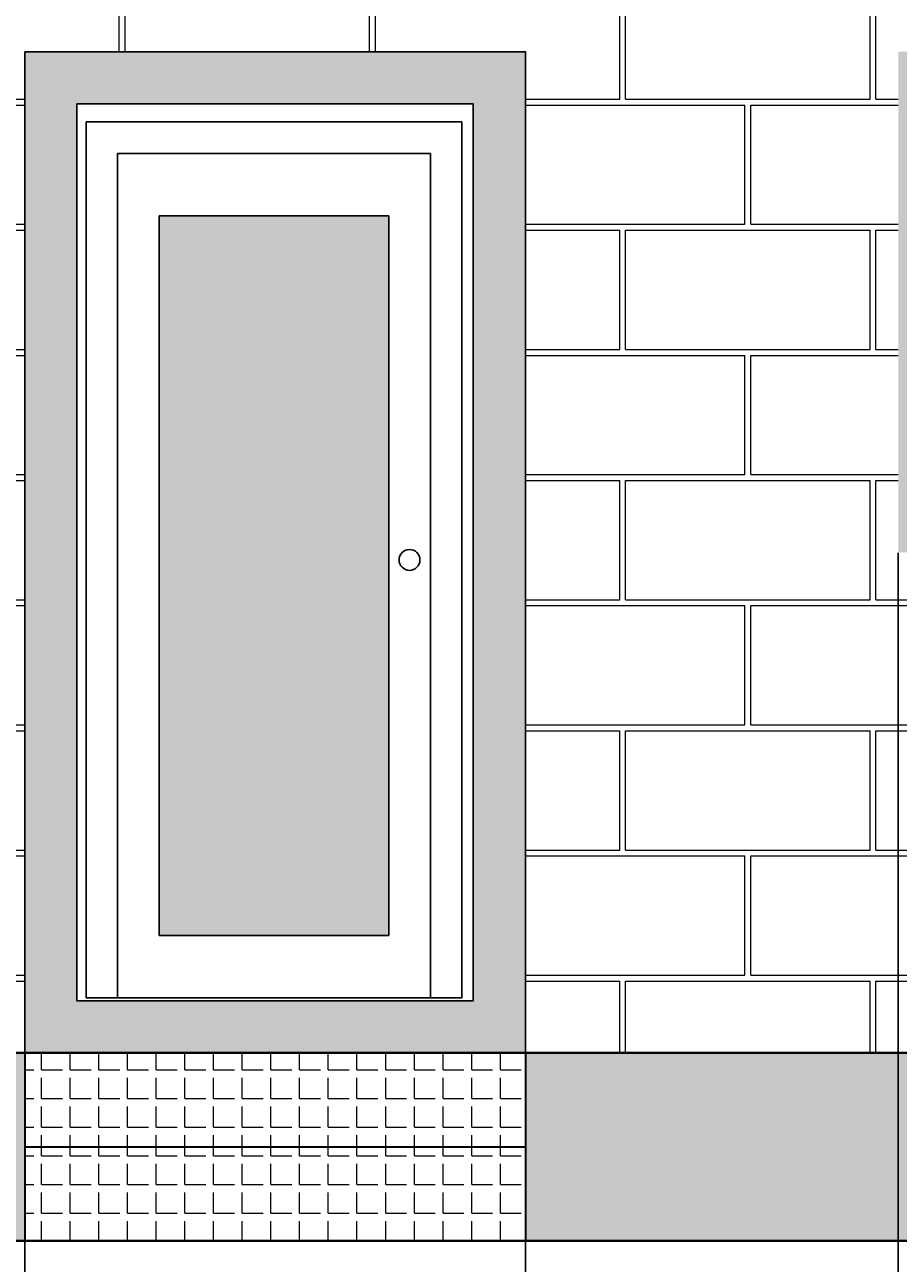
# Model space of a CAD drawing. Units: inches. Extents: x -301 to 715, y -607 to 364.
# Tile 135 of 141: x 413 to 497, y -510 to -391. Entities that reach past the tile are written whole.
import ezdxf

# ---------------------------------------------------------------- set-up
doc = ezdxf.new("R2010")
doc.units = ezdxf.units.IN
doc.header["$MEASUREMENT"] = 0
for name, color, linetype, lineweight in [('A-ANNO-DIMS', 2, 'Continuous', 18), ('A-DOOR', 4, 'Continuous', 25), ('A-ELEV', 220, 'Continuous', 30), ('A-ELEV-PATT', 4, 'Continuous', 13)]:
    doc.layers.add(name, color=color, linetype=linetype, lineweight=lineweight)
doc.styles.get("Standard").update_dxf_attribs({"font": 'arial.ttf'})
doc.dimstyles.get("Standard").update_dxf_attribs({"dimtxt": 0.18, "dimasz": 0.18, "dimexe": 0.18, "dimexo": 0.0625, "dimgap": 0.09, "dimtad": 0, "dimtih": 1, "dimtoh": 1, "dimdec": 1, "dimzin": 0, "dimdsep": 46, "dimlunit": 4, "dimtxsty": 'Standard', "dimcen": 0.09, "dimclrd": 3, "dimclre": 4, "dimclrt": 6, "dimadec": 0, "dimazin": 0, "dimtfac": 1, "dimtdec": 1, "dimtofl": 0, "dimtmove": 0, "dimatfit": 3, "dimfxl": 1, "dimtfill": 2, "dimtfillclr": 51, "dimtolj": 1, "dimtzin": 0, "dimarcsym": 0})

# ---------------------------------------------------------------- blocks, each defined once
blk = doc.blocks.new('*U31')
blk.add_lwpolyline([(3.12, 0.01), (0.12, 0.01), (0.12, 84.01), (36.12, 84.01), (36.12, 0.01), (33.12, 0.01)])
for points in [[(33.12, 80.99), (33.12, 0.01), (3.12, 0.01), (3.12, 80.99)], [(29.12, 6.01), (29.12, 74.99), (7.12, 74.99), (7.12, 6.01)]]:
    blk.add_lwpolyline(points, close=True)
blk.add_circle((31.12, 42.01), 1)
blk = doc.blocks.new('*D197')
at = {"layer": 'A-ANNO-DIMS', "color": 4, "lineweight": -2, "transparency": 16777216}
for p, q in [((413.02, -489.61), (413.02, -606.79)), ((461.02, -489.61), (461.02, -606.79))]:
    blk.add_line(p, q, dxfattribs=at)
at = {"layer": 'A-ANNO-DIMS', "color": 3, "lineweight": -2, "transparency": 16777216}
for p, q in [((413.2, -606.61), (436.68, -606.61)), ((460.84, -606.61), (437.35, -606.61))]:
    blk.add_line(p, q, dxfattribs=at)
at = {"layer": 'A-ANNO-DIMS', "color": 3, "transparency": 16777216}
for points in [[(413.2, -606.58), (413.2, -606.64), (413.02, -606.61)], [(460.84, -606.58), (460.84, -606.64), (461.02, -606.61)]]:
    blk.add_solid(points, dxfattribs=at)
at = {"layer": 'Defpoints', "color": 0, "transparency": 16777216}
for p in [(413.02, -489.55), (461.02, -489.55), (461.02, -606.61)]:
    blk.add_point(p, dxfattribs=at)
at = {"layer": 'A-ANNO-DIMS', "color": 6, "transparency": 16777216, "insert": (437.02, -606.61), "char_height": 0.18, "attachment_point": 5, "bg_fill": 1, "box_fill_scale": 1.25, "bg_fill_color": 51, "bg_fill_transparency": 0}
blk.add_mtext('\\A1;4\'-0"', dxfattribs=at)
blk = doc.blocks.new('*D198')
at = {"layer": 'A-ANNO-DIMS', "color": 4, "lineweight": -2, "transparency": 16777216}
for p, q in [((496.77, -441.61), (496.77, -606.79)), ((461.02, -489.61), (461.02, -606.79))]:
    blk.add_line(p, q, dxfattribs=at)
at = {"layer": 'A-ANNO-DIMS', "color": 3, "lineweight": -2, "transparency": 16777216}
for p, q in [((461.2, -606.61), (478.56, -606.61)), ((496.59, -606.61), (479.22, -606.61))]:
    blk.add_line(p, q, dxfattribs=at)
at = {"layer": 'A-ANNO-DIMS', "color": 3, "transparency": 16777216}
for points in [[(461.2, -606.58), (461.2, -606.64), (461.02, -606.61)], [(496.59, -606.58), (496.59, -606.64), (496.77, -606.61)]]:
    blk.add_solid(points, dxfattribs=at)
at = {"layer": 'Defpoints', "color": 0, "transparency": 16777216}
for p in [(496.77, -441.55), (461.02, -489.55), (496.77, -606.61)]:
    blk.add_point(p, dxfattribs=at)
at = {"layer": 'A-ANNO-DIMS', "color": 6, "transparency": 16777216, "insert": (478.89, -606.61), "char_height": 0.18, "attachment_point": 5, "bg_fill": 1, "box_fill_scale": 1.25, "bg_fill_color": 51, "bg_fill_transparency": 0}
blk.add_mtext('\\A1;3\'-0"', dxfattribs=at)

msp = doc.modelspace()

# ---------------------------------------------------------------- hatches: boundary and pattern name
at = {"layer": 'A-ELEV-PATT'}
h = msp.add_hatch(color=256, dxfattribs=at)
h.dxf.hatch_style = 1
h.paths.add_polyline_path([(591.52, -363.55), (254.02, -363.55), (254.02, -369.55), (591.52, -369.55)])
h.paths.add_polyline_path([(461.02, -393.55), (413.02, -393.55), (413.02, -489.55), (461.02, -489.55)])
h.paths.add_polyline_path([(456.02, -398.55), (456.02, -484.55), (418.02, -484.55), (418.02, -398.55)], flags=16)
h.paths.add_polyline_path([(546.77, -393.55), (496.77, -393.55), (496.77, -441.55), (546.77, -441.55)])
h.paths.add_polyline_path([(501.77, -398.55), (541.77, -398.55), (541.77, -436.55), (501.77, -436.55)], flags=16)
h.paths.add_polyline_path([(360.02, -393.55), (310.02, -393.55), (310.02, -441.55), (360.02, -441.55)])
h.paths.add_polyline_path([(355.02, -398.55), (355.02, -436.55), (315.02, -436.55), (315.02, -398.55)], flags=16)
h = msp.add_hatch(dxfattribs=at)
h.set_pattern_fill('AR-B816C', color=256, scale=1.5)
h.set_pattern_definition([(0, (458.621, 9.325), (12, 12), [23.4375, -0.5625]), (0, (446.621, 9.887), (12, 12), [23.4375, -0.5625]), (90, (458.621, 9.325), (-12, 12), [-12.5625, 11.4375]), (90, (458.059, 9.325), (-12, 12), [-12.5625, 11.4375])])
h.paths.add_polyline_path([(254.02, -489.55), (413.02, -489.55), (413.02, -393.55), (461.02, -393.55), (461.02, -489.55), (591.52, -489.55), (591.52, -369.55), (254.02, -369.55)])
h.paths.add_polyline_path([(310.02, -393.55), (360.02, -393.55), (360.02, -441.55), (310.02, -441.55)], flags=16)
h.paths.add_polyline_path([(315.02, -398.55), (355.02, -398.55), (355.02, -436.55), (315.02, -436.55)], flags=0)
h.paths.add_polyline_path([(496.77, -393.55), (546.77, -393.55), (546.77, -441.55), (496.77, -441.55)], flags=16)
h.paths.add_polyline_path([(501.77, -398.55), (541.77, -398.55), (541.77, -436.55), (501.77, -436.55)], flags=0)
h = msp.add_hatch(color=256, dxfattribs=at)
h.dxf.hatch_style = 1
h.paths.add_polyline_path([(425.92, -478.28), (447.92, -478.28), (447.92, -409.3), (425.92, -409.3)])
h = msp.add_hatch(dxfattribs=at)
h.set_pattern_fill('AR-CONC', color=256, scale=2)
h.set_pattern_definition([(50, (458.621, 9.325), (14.3452, -1.25504), [1.5, -16.5]), (355, (458.621, 9.325), (-2.77503, 15.04384), [1.2, -13.2]), (100.4514, (459.817, 9.22), (11.57018, 13.7888), [1.2748, -14.02284]), (46.1842, (458.621, 13.325), (21.3448, -3.3104), [2.25, -24.75]), (96.6356, (460.4, 13.049), (18.69324, 19.4824), [1.9122, -21.0343]), (351.184, (458.62, 13.325), (18.6932, 19.4824), [1.8, -19.8]), (21, (460.621, 12.325), (11.93814, -8.05238), [1.5, -16.5]), (326, (460.621, 12.325), (4.8663, 14.503), [1.2, -13.2]), (71.4514, (461.616, 11.654), (16.80445, 6.45062), [1.2748, -14.02284]), (37.5, (458.621, 9.325), (0.243197, 6.657877), [0, -13.04, 0, -13.4, 0, -13.25]), (7.5, (458.621, 9.325), (5.26139, 7.88823), [0, -7.64, 0, -12.74, 0, -5.05]), (327.5, (454.161, 9.325), (10.67645, -0.4511), [0, -5, 0, -15.6, 0, -20.7]), (317.5, (452.161, 9.325), (11.66372, 2.0021), [0, -6.5, 0, -10.36, 0, -14.7])])
h.paths.add_polyline_path([(254.02, -489.55), (254.02, -507.55), (413.02, -507.55), (413.02, -489.55)])
h.paths.add_polyline_path([(591.52, -507.55), (591.52, -489.55), (461.02, -489.55), (461.02, -507.55)])
h = msp.add_hatch(dxfattribs=at)
h.set_pattern_fill('ANGLE', color=256, scale=10)
h.set_pattern_definition([(0, (458.621, 9.3248), (0, 2.75), [2, -0.75]), (90, (458.621, 9.3248), (-2.75, 2e-16), [2, -0.75])])
h.paths.add_polyline_path([(461.02, -489.55), (413.02, -489.55), (413.02, -498.55), (461.02, -498.55)])
h.paths.add_polyline_path([(461.02, -498.55), (413.02, -498.55), (413.02, -507.55), (461.02, -507.55)])

# ---------------------------------------------------------------- linework, layer by layer
at = {"layer": 'A-DOOR'}
for points in [[(413.02, -393.55), (461.02, -393.55), (461.02, -489.55), (413.02, -489.55)], [(418.02, -398.55), (456.02, -398.55), (456.02, -484.55), (418.02, -484.55)]]:
    msp.add_lwpolyline(points, close=True, dxfattribs=at)
at = {"layer": 'A-ELEV'}
for p, q in [((254.02, -489.55), (591.52, -489.55)), ((413.02, -489.55), (413.02, -507.55)), ((413.02, -489.55), (461.02, -489.55)), ((461.02, -489.55), (461.02, -507.55)), ((413.02, -498.55), (461.02, -498.55)), ((254.02, -507.55), (591.52, -507.55))]:
    msp.add_line(p, q, dxfattribs=at)
for points in [[(254.02, -369.55), (591.52, -369.55), (591.52, -489.55), (254.02, -489.55)], [(254.02, -489.55), (591.52, -489.55), (591.52, -507.55), (254.02, -507.55)]]:
    msp.add_lwpolyline(points, close=True, dxfattribs=at)

# ---------------------------------------------------------------- block references
at = {"layer": 'A-DOOR'}
msp.add_blockref('*U31', (418.79, -484.29), dxfattribs=at)

# ---------------------------------------------------------------- dimensions: what is measured, and where the dimension line sits
at = {"layer": 'A-ANNO-DIMS'}
for base, p1, p2, picture, middle in [((496.767813, -606.608725), (461.017813, -489.55247), (496.767813, -441.55247), '*D198', (478.892813, -606.608725)), ((461.02, -606.61), (413.02, -489.55), (461.02, -489.55), '*D197', (437.02, -606.61))]:
    dim = msp.add_linear_dim(base=base, p1=p1, p2=p2, dimstyle='Standard', override={"dimdec": 1, "dimlfac": 1, "dimrnd": 0, "dimzin": 1, "dimdsep": 46, "dimlunit": 4, "dimfrac": 2}, dxfattribs=at)
    dim.commit()
    dim.dimension.update_dxf_attribs({"geometry": picture, "text_midpoint": middle})

doc.saveas('drawing.dxf')
